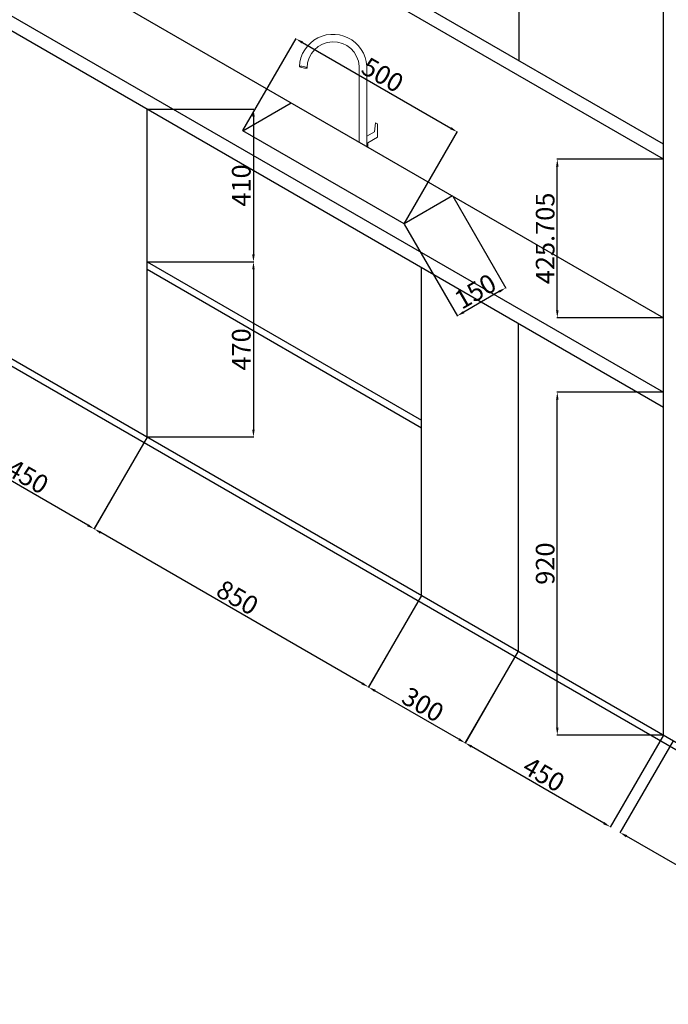
# Model space of a CAD drawing. Units: centimetres. Extents: x 209356 to 217348, y 253987 to 259034.
# Tile 4 of 7: x 212337 to 214078, y 254619 to 257262. Entities that reach past the tile are written whole.
import ezdxf

# ---------------------------------------------------------------- set-up
doc = ezdxf.new("R2010")
doc.units = ezdxf.units.CM
for name, color, linetype, lineweight in [('A-ANNO-DIMS', 2, 'Continuous', 18), ('A-ELEV', 7, 'Continuous', 25), ('A-FLOR-FIXT', 8, 'Continuous', 18)]:
    doc.layers.add(name, color=color, linetype=linetype, lineweight=lineweight)
doc.styles.get("Standard").update_dxf_attribs({"font": 'arial.ttf'})
doc.dimstyles.new('ISO-25', dxfattribs={"dimtxt": 50, "dimasz": 20, "dimexe": 1.25, "dimexo": 0.625, "dimtad": 1, "dimdec": 1, "dimtxsty": 'Standard', "dimcen": 2.5, "dimadec": 0, "dimazin": 0, "dimtfac": 1, "dimtdec": 1, "dimtmove": 0, "dimatfit": 3, "dimfxl": 1, "dimarcsym": 0})

# ---------------------------------------------------------------- blocks, each defined once
blk = doc.blocks.new('TAP')
for p, q in [((213588.6, 256736.5), (213588.6, 256940)), ((213609, 256724.8), (213609, 256928.3)), ((213632.8, 256788.1), (213629.4, 256764)), ((213638, 256785.1), (213632.8, 256788.1)), ((213638, 256749.8), (213638, 256785.1)), ((213609, 256752.2), (213629.4, 256764)), ((213638, 256749.8), (213638, 256759.8)), ((213612, 256734.8), (213638, 256749.8)), ((213612, 256724.8), (213612, 256734.8)), ((213609, 256724.8), (213612, 256724.8))]:
    blk.add_line(p, q)
for centre, radius, start, end in [((213518.6, 256935.1), 90.6, 355.6958, 177.4424), ((213518.8, 256935.8), 70, 3.4473, 180.1774)]:
    blk.add_arc(centre, radius, start, end)
blk.add_ellipse((213438.4, 256937.4), major_axis=(10.4, -1.7), ratio=0.185071)
blk = doc.blocks.new('*D15')
at = {"layer": 'A-ANNO-DIMS', "color": 0, "lineweight": -2, "transparency": 16777216}
for p, q in [((212289.3, 256366), (212146.4, 256118.6)), ((212679, 256141), (212536.2, 255893.6)), ((212519.5, 255904.7), (212164.4, 256109.7))]:
    blk.add_line(p, q, dxfattribs=at)
at = {"layer": 'A-ANNO-DIMS', "color": 0, "transparency": 16777216}
for points in [[(212166.1, 256112.6), (212162.7, 256106.8), (212147.1, 256119.7)], [(212521.1, 255907.6), (212517.8, 255901.8), (212536.8, 255894.7)]]:
    blk.add_solid(points, dxfattribs=at)
at = {"layer": 'Defpoints', "color": 0, "transparency": 16777216}
for p in [(212289.6, 256366.5), (212679.3, 256141.5), (212147.1, 256119.7)]:
    blk.add_point(p, dxfattribs=at)
at = {"layer": 'A-ANNO-DIMS', "color": 0, "transparency": 16777216, "insert": (212355, 256029.9), "char_height": 50, "attachment_point": 5, "rotation": 330}
blk.add_mtext('450', dxfattribs=at)
blk = doc.blocks.new('*D16')
at = {"layer": 'A-ANNO-DIMS', "color": 0, "lineweight": -2, "transparency": 16777216}
for p, q in [((212679, 256141), (212536.3, 255893.6)), ((213256, 255480), (212554.2, 255884.7)), ((213415.3, 255716.4), (213272.7, 255469))]:
    blk.add_line(p, q, dxfattribs=at)
at = {"layer": 'A-ANNO-DIMS', "color": 0, "transparency": 16777216}
for points in [[(212555.9, 255887.6), (212552.6, 255881.8), (212536.9, 255894.7)], [(213257.6, 255482.9), (213254.3, 255477.2), (213273.3, 255470.1)]]:
    blk.add_solid(points, dxfattribs=at)
at = {"layer": 'Defpoints', "color": 0, "transparency": 16777216}
for p in [(212679.3, 256141.5), (212536.9, 255894.7), (213415.6, 255717)]:
    blk.add_point(p, dxfattribs=at)
at = {"layer": 'A-ANNO-DIMS', "color": 0, "transparency": 16777216, "insert": (212918.2, 255705), "char_height": 50, "attachment_point": 5, "rotation": 330.0318}
blk.add_mtext('850', dxfattribs=at)
blk = doc.blocks.new('*D17')
at = {"layer": 'A-ANNO-DIMS', "color": 0, "lineweight": -2, "transparency": 16777216}
for p, q in [((213415.3, 255716.4), (213272.5, 255469.1)), ((213675.1, 255566.4), (213532.3, 255319.1)), ((213515.6, 255330.1), (213290.5, 255460.1))]:
    blk.add_line(p, q, dxfattribs=at)
at = {"layer": 'A-ANNO-DIMS', "color": 0, "transparency": 16777216}
for points in [[(213292.1, 255463), (213288.8, 255457.3), (213273.1, 255470.1)], [(213517.3, 255333), (213514, 255327.3), (213532.9, 255320.1)]]:
    blk.add_solid(points, dxfattribs=at)
at = {"layer": 'Defpoints', "color": 0, "transparency": 16777216}
for p in [(213415.6, 255717), (213675.4, 255567), (213273.1, 255470.1)]:
    blk.add_point(p, dxfattribs=at)
at = {"layer": 'A-ANNO-DIMS', "color": 0, "transparency": 16777216, "insert": (213416.1, 255417.8), "char_height": 50, "attachment_point": 5, "rotation": 330}
blk.add_mtext('300', dxfattribs=at)
blk = doc.blocks.new('*D18')
at = {"layer": 'A-ANNO-DIMS', "color": 0, "lineweight": -2, "transparency": 16777216}
for p, q in [((213675.1, 255566.4), (213532.1, 255319.2)), ((214064.6, 255341), (213921.5, 255093.8)), ((213904.9, 255104.9), (213550, 255310.3))]:
    blk.add_line(p, q, dxfattribs=at)
at = {"layer": 'A-ANNO-DIMS', "color": 0, "transparency": 16777216}
for points in [[(213551.7, 255313.2), (213548.3, 255307.4), (213532.7, 255320.3)], [(213906.5, 255107.8), (213903.2, 255102), (213922.2, 255094.9)]]:
    blk.add_solid(points, dxfattribs=at)
at = {"layer": 'Defpoints', "color": 0, "transparency": 16777216}
for p in [(213675.4, 255567), (214064.9, 255341.5), (213532.7, 255320.3)]:
    blk.add_point(p, dxfattribs=at)
at = {"layer": 'A-ANNO-DIMS', "color": 0, "transparency": 16777216, "insert": (213740.5, 255230.2), "char_height": 50, "attachment_point": 5, "rotation": 329.9399}
blk.add_mtext('450', dxfattribs=at)
blk = doc.blocks.new('*D19')
at = {"layer": 'A-ANNO-DIMS', "color": 0, "lineweight": -2, "transparency": 16777216}
for p, q in [((212679.9, 257021.5), (212965.5, 257021.5)), ((212964.3, 257001.5), (212964.3, 256631.5)), ((212679.9, 256611.5), (212965.5, 256611.5))]:
    blk.add_line(p, q, dxfattribs=at)
at = {"layer": 'A-ANNO-DIMS', "color": 0, "transparency": 16777216}
for points in [[(212960.9, 257001.5), (212967.6, 257001.5), (212964.3, 257021.5)], [(212960.9, 256631.5), (212967.6, 256631.5), (212964.3, 256611.5)]]:
    blk.add_solid(points, dxfattribs=at)
at = {"layer": 'Defpoints', "color": 0, "transparency": 16777216}
for p in [(212679.3, 257021.5), (212679.3, 256611.5), (212964.3, 256611.5)]:
    blk.add_point(p, dxfattribs=at)
at = {"layer": 'A-ANNO-DIMS', "color": 0, "transparency": 16777216, "insert": (212938.1, 256816.5), "char_height": 50, "attachment_point": 5, "rotation": 90}
blk.add_mtext('410', dxfattribs=at)
blk = doc.blocks.new('*D20')
at = {"layer": 'A-ANNO-DIMS', "color": 0, "lineweight": -2, "transparency": 16777216}
for p, q in [((212679.9, 256611.5), (212965.5, 256611.5)), ((212964.3, 256591.5), (212964.3, 256161.5)), ((212679.9, 256141.5), (212965.5, 256141.5))]:
    blk.add_line(p, q, dxfattribs=at)
at = {"layer": 'A-ANNO-DIMS', "color": 0, "transparency": 16777216}
for points in [[(212960.9, 256591.5), (212967.6, 256591.5), (212964.3, 256611.5)], [(212960.9, 256161.5), (212967.6, 256161.5), (212964.3, 256141.5)]]:
    blk.add_solid(points, dxfattribs=at)
at = {"layer": 'Defpoints', "color": 0, "transparency": 16777216}
for p in [(212679.3, 256611.5), (212679.3, 256141.5), (212964.3, 256141.5)]:
    blk.add_point(p, dxfattribs=at)
at = {"layer": 'A-ANNO-DIMS', "color": 0, "transparency": 16777216, "insert": (212938.1, 256376.5), "char_height": 50, "attachment_point": 5, "rotation": 90}
blk.add_mtext('470', dxfattribs=at)
blk = doc.blocks.new('*D23')
at = {"layer": 'A-ANNO-DIMS', "color": 0, "lineweight": -2, "transparency": 16777216}
for p, q in [((214064.3, 256887.3), (213778.7, 256887.3)), ((213779.9, 256481.5), (213779.9, 256867.3)), ((214064.3, 256461.5), (213778.7, 256461.5))]:
    blk.add_line(p, q, dxfattribs=at)
at = {"layer": 'A-ANNO-DIMS', "color": 0, "transparency": 16777216}
for points in [[(213776.6, 256867.3), (213783.3, 256867.3), (213779.9, 256887.3)], [(213776.6, 256481.5), (213783.3, 256481.5), (213779.9, 256461.5)]]:
    blk.add_solid(points, dxfattribs=at)
at = {"layer": 'Defpoints', "color": 0, "transparency": 16777216}
for p in [(213779.9, 256887.3), (214064.9, 256887.3), (214064.9, 256461.5)]:
    blk.add_point(p, dxfattribs=at)
at = {"layer": 'A-ANNO-DIMS', "color": 0, "transparency": 16777216, "insert": (213753.8, 256674.4), "char_height": 50, "attachment_point": 5, "rotation": 90}
blk.add_mtext('425.705', dxfattribs=at)
blk = doc.blocks.new('*D24')
at = {"layer": 'A-ANNO-DIMS', "color": 0, "lineweight": -2, "transparency": 16777216}
for p, q in [((212936.2, 256964), (213079, 257211.3)), ((213095.7, 257200.2), (213494, 256970.2)), ((213369.2, 256714), (213512, 256961.3))]:
    blk.add_line(p, q, dxfattribs=at)
at = {"layer": 'A-ANNO-DIMS', "color": 0, "transparency": 16777216}
for points in [[(213097.3, 257203.1), (213094, 257197.4), (213078.3, 257210.2)], [(213495.7, 256973.1), (213492.4, 256967.4), (213511.4, 256960.2)]]:
    blk.add_solid(points, dxfattribs=at)
at = {"layer": 'Defpoints', "color": 0, "transparency": 16777216}
for p in [(212935.8, 256963.4), (213511.4, 256960.2), (213368.9, 256713.4)]:
    blk.add_point(p, dxfattribs=at)
at = {"layer": 'A-ANNO-DIMS', "color": 0, "transparency": 16777216, "insert": (213307.9, 257107.9), "char_height": 50, "attachment_point": 5, "rotation": 330}
blk.add_mtext('500', dxfattribs=at)
blk = doc.blocks.new('*D25')
at = {"layer": 'A-ANNO-DIMS', "color": 0, "lineweight": -2, "transparency": 16777216}
for p, q in [((213499.1, 256787.9), (213641.9, 256540.5)), ((213369.2, 256712.9), (213512, 256465.5)), ((213623.9, 256531.6), (213528.7, 256476.6))]:
    blk.add_line(p, q, dxfattribs=at)
at = {"layer": 'A-ANNO-DIMS', "color": 0, "transparency": 16777216}
for points in [[(213622.3, 256534.5), (213625.6, 256528.7), (213641.3, 256541.6)], [(213527, 256479.5), (213530.3, 256473.7), (213511.4, 256466.6)]]:
    blk.add_solid(points, dxfattribs=at)
at = {"layer": 'Defpoints', "color": 0, "transparency": 16777216}
for p in [(213498.8, 256788.4), (213368.9, 256713.4), (213511.4, 256466.6)]:
    blk.add_point(p, dxfattribs=at)
at = {"layer": 'A-ANNO-DIMS', "color": 0, "transparency": 16777216, "insert": (213563.2, 256526.8), "char_height": 50, "attachment_point": 5, "rotation": 30}
blk.add_mtext('150', dxfattribs=at)
blk = doc.blocks.new('*D26')
at = {"layer": 'A-ANNO-DIMS', "color": 0, "lineweight": -2, "transparency": 16777216}
for p, q in [((214064.3, 256261.5), (213778.7, 256261.5)), ((213779.9, 255361.5), (213779.9, 256241.5)), ((214064.3, 255341.5), (213778.7, 255341.5))]:
    blk.add_line(p, q, dxfattribs=at)
at = {"layer": 'A-ANNO-DIMS', "color": 0, "transparency": 16777216}
for points in [[(213776.6, 256241.5), (213783.3, 256241.5), (213779.9, 256261.5)], [(213776.6, 255361.5), (213783.3, 255361.5), (213779.9, 255341.5)]]:
    blk.add_solid(points, dxfattribs=at)
at = {"layer": 'Defpoints', "color": 0, "transparency": 16777216}
for p in [(213779.9, 256261.5), (214064.9, 256261.5), (214064.9, 255341.5)]:
    blk.add_point(p, dxfattribs=at)
at = {"layer": 'A-ANNO-DIMS', "color": 0, "transparency": 16777216, "insert": (213753.8, 255801.5), "char_height": 50, "attachment_point": 5, "rotation": 90}
blk.add_mtext('920', dxfattribs=at)
blk = doc.blocks.new('*D27')
at = {"layer": 'A-ANNO-DIMS', "color": 0, "lineweight": -2, "transparency": 16777216}
for p, q in [((214090.6, 255326), (213947.8, 255078.6)), ((214727.8, 254629.7), (213965.7, 255069.7)), ((214887.3, 254866), (214744.5, 254618.6))]:
    blk.add_line(p, q, dxfattribs=at)
at = {"layer": 'A-ANNO-DIMS', "color": 0, "transparency": 16777216}
for points in [[(213967.4, 255072.6), (213964.1, 255066.8), (213948.4, 255079.7)], [(214729.5, 254632.6), (214726.2, 254626.8), (214745.1, 254619.7)]]:
    blk.add_solid(points, dxfattribs=at)
at = {"layer": 'Defpoints', "color": 0, "transparency": 16777216}
for p in [(214090.9, 255326.5), (213948.4, 255079.7), (214887.6, 254866.5)]:
    blk.add_point(p, dxfattribs=at)
at = {"layer": 'A-ANNO-DIMS', "color": 0, "transparency": 16777216, "insert": (214359.9, 254872.4), "char_height": 50, "attachment_point": 5, "rotation": 330}
blk.add_mtext('920', dxfattribs=at)

msp = doc.modelspace()

# ---------------------------------------------------------------- linework, layer by layer
at = {"layer": 'A-ELEV'}
for p, q in [((214064.9209, 255341.5492), (214064.9209, 257741.5492)), ((213677.037, 257671.1985), (213677.037, 257151.1985)), ((212289.5688, 257486.5492), (214064.9209, 256461.5492)), ((214064.9209, 256927.2537), (213192.0627, 257431.1985)), ((214064.9209, 256887.2537), (213157.4217, 257411.1985)), ((212289.5688, 257286.5492), (214064.9209, 256261.5492)), ((212289.5688, 257246.5492), (214064.9209, 256221.5492)), ((212935.8421, 256963.4231), (213065.7459, 257038.4231)), ((212679.2802, 256141.5492), (212679.2802, 257021.5492)), ((213368.8548, 256713.4231), (212935.8421, 256963.4231)), ((213498.7586, 256788.4231), (213368.8548, 256713.4231)), ((212679.2802, 256611.5492), (213415.6415, 256186.4107)), ((212679.2802, 256591.5492), (213415.6415, 256166.4107)), ((213415.6415, 255716.9555), (213415.6415, 256596.9555)), ((213502.2441, 256546.4107), (213502.2441, 256546.9555)), ((213675.4492, 255566.9555), (213675.4492, 256446.9555)), ((212289.5688, 256366.5492), (214887.645, 254866.5492)), ((212289.5688, 256346.5492), (214887.645, 254846.5492)), ((214064.9209, 255341.5492), (214064.9209, 256221.5492))]:
    msp.add_line(p, q, dxfattribs=at)

# ---------------------------------------------------------------- block references
at = {"layer": 'A-FLOR-FIXT'}
msp.add_blockref('TAP', (-340.5399, 196.6108), dxfattribs=at)

# ---------------------------------------------------------------- dimensions: what is measured, and where the dimension line sits
at = {"layer": 'A-ANNO-DIMS'}
for base, p1, p2, angle, override, picture, middle in [((213511.3548, 256960.2403), (212935.8421, 256963.4231), (213368.8548, 256713.4231), 330, {"dimdec": 0, "dimlfac": 1, "dimrnd": 0, "dimzin": 0, "dimdsep": 46, "dimlunit": 2}, '*D24', (213307.9253, 257107.89)), ((212964.2802, 256611.5492), (212679.2802, 257021.5492), (212679.2802, 256611.5492), 270, {"dimdec": 0, "dimlfac": 1, "dimrnd": 0, "dimzin": 0, "dimdsep": 46, "dimlunit": 2}, '*D19', (212938.1266, 256816.5492)), ((213779.9208630003, 256887.2536530002), (214064.920863, 256461.5491530001), (214064.920863, 256887.253653), 90, {"dimdec": 3, "dimlfac": 1, "dimrnd": 0, "dimzin": 0, "dimdsep": 46, "dimlunit": 2}, '*D23', (213753.7672136142, 256674.401403)), ((213511.3548, 256466.6058), (213498.7586, 256788.4231), (213368.8548, 256713.4231), 210, {"dimdec": 0, "dimlfac": 1, "dimrnd": 0, "dimzin": 0, "dimdsep": 46, "dimlunit": 2}, '*D25', (213563.2299, 256526.7556)), ((212964.2802, 256141.5492), (212679.2802, 256611.5492), (212679.2802, 256141.5492), 270, {"dimdec": 0, "dimlfac": 1, "dimrnd": 0, "dimzin": 0, "dimdsep": 46, "dimlunit": 2}, '*D20', (212938.1266, 256376.5492)), ((212147.0688, 256119.7319), (212679.2802, 256141.5492), (212289.5688, 256366.5492), 150, {"dimdec": 0, "dimlfac": 1, "dimrnd": 0, "dimzin": 0, "dimdsep": 46, "dimlunit": 2}, '*D15', (212355.0013, 256029.8816)), ((213779.9209, 256261.5492), (214064.9209, 255341.5492), (214064.9209, 256261.5492), 90, {"dimdec": 0, "dimlfac": 1, "dimrnd": 0, "dimzin": 0, "dimdsep": 46, "dimlunit": 2}, '*D26', (213753.7672, 255801.5492)), ((212536.9172, 255894.6529), (213415.6415, 255716.9555), (212679.2802, 256141.5492), 150.0317987, {"dimdec": 0, "dimlfac": 1, "dimrnd": 0, "dimzin": 0, "dimdsep": 46, "dimlunit": 2}, '*D16', (212918.1621, 255705.013)), ((213273.1415, 255470.1382), (213675.4492, 255566.9555), (213415.6415, 255716.9555), 150, {"dimdec": 0, "dimlfac": 1, "dimrnd": 0, "dimzin": 0, "dimdsep": 46, "dimlunit": 2}, '*D17', (213416.1307, 255417.8027)), ((213532.6905, 255320.2878), (214064.9209, 255341.5492), (213675.4492, 255566.9555), 149.9399349, {"dimdec": 0, "dimlfac": 1, "dimrnd": 0, "dimzin": 0, "dimdsep": 46, "dimlunit": 2}, '*D18', (213740.5269, 255230.2206)), ((213948.4016, 255079.7319), (214887.645, 254866.5492), (214090.9016, 255326.5492), 150, {"dimdec": 0, "dimlfac": 1, "dimrnd": 0, "dimzin": 0, "dimdsep": 46, "dimlunit": 2}, '*D27', (214359.8501, 254872.3816))]:
    dim = msp.add_linear_dim(base=base, p1=p1, p2=p2, angle=angle, dimstyle='ISO-25', override=override, dxfattribs=at)
    dim.commit()
    dim.dimension.update_dxf_attribs({"geometry": picture, "text_midpoint": middle})

doc.saveas('drawing.dxf')
